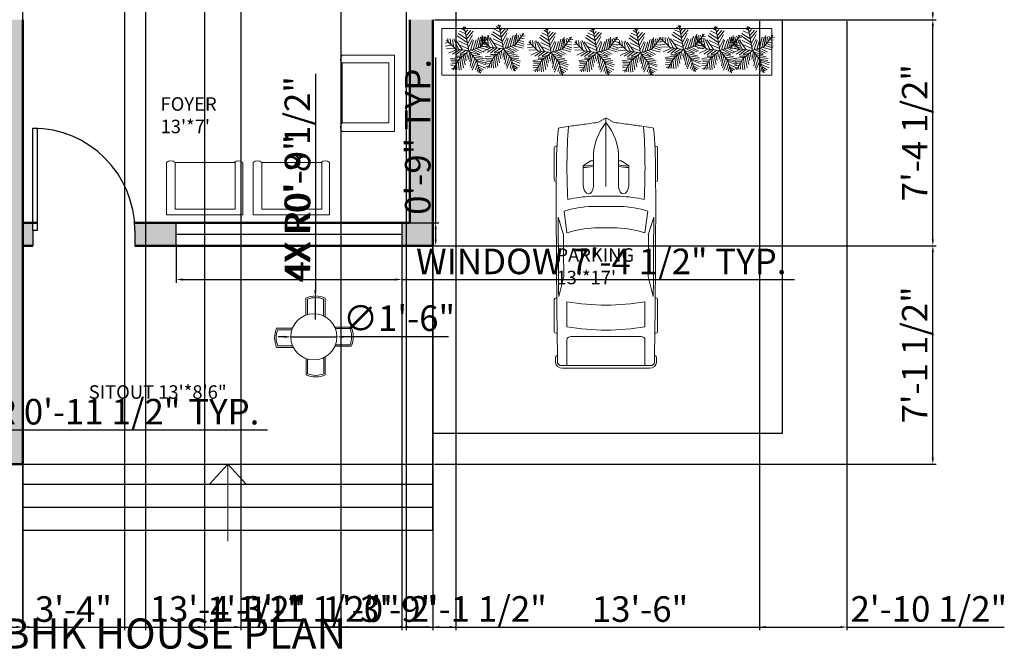
# Model space of a CAD drawing. Units: inches. Extents: x 772 to 1415, y 1573 to 2261.
# Tile 2 of 4: x 984 to 1369, y 1573 to 1820. Entities that reach past the tile are written whole.
import ezdxf

# ---------------------------------------------------------------- set-up
doc = ezdxf.new("R2010")
doc.units = ezdxf.units.IN
for name, color, linetype, lineweight in [('A-ANNO-DIMS', 2, 'Continuous', 18), ('A-ANNO-SYMB', 7, 'Continuous', 18), ('A-ANNO-TEXT', 10, 'Continuous', 25), ('A-AREA-IDEN', 10, 'Continuous', 25), ('A-EQPM-VEH', 8, 'Continuous', 13), ('A-FLOR-EDGE', 7, 'Continuous', 25), ('A-FLOR-STRS', 7, 'Continuous', 25), ('A-WALL-PATT', 140, 'Continuous', 13), ('DOOR', 52, 'Continuous', 25), ('FUR', 210, 'Continuous', 18), ('L-PLNT-BEDS', 92, 'Continuous', 18), ('TREE', 92, 'Continuous', 13), ('WALL', 7, 'Continuous', 50), ('WINDOW', 80, 'Continuous', 25)]:
    doc.layers.add(name, color=color, linetype=linetype, lineweight=lineweight)
doc.styles.get("Standard").update_dxf_attribs({"font": 'arial.ttf'})
doc.dimstyles.new('ISO-25', dxfattribs={"dimtxt": 10, "dimasz": 2.5, "dimexe": 1.25, "dimexo": 0.625, "dimtad": 1, "dimdec": 0, "dimlunit": 4, "dimtxsty": 'Standard', "dimcen": 2.5, "dimadec": 0, "dimazin": 0, "dimtfac": 1, "dimtdec": 0, "dimtmove": 0, "dimatfit": 3, "dimfxl": 1, "dimarcsym": 0})

# ---------------------------------------------------------------- blocks, each defined once
blk = doc.blocks.new('*U2')
for p, q in [((0, 0), (0, -6)), ((40, 0), (40, -6))]:
    blk.add_line(p, q)
blk.add_lwpolyline([(0, 0), (0, 40), (1.75, 40), (1.75, 0)], close=True)
blk.add_arc((0, 0), 40, 0, 90)
blk = doc.blocks.new('*U6')
for p, q in [((-7.288, 39.707), (-21.778, 46.673)), ((-8.737, 47.138), (-17.069, 52.711)), ((-10.186, 53.64), (-13.084, 55.962)), ((0, 0), (-10.5, 57)), ((-9.099, 51.782), (-6.563, 55.962)), ((-7.65, 43.423), (-2.578, 49.46)), ((-5.839, 35.992), (4.667, 48.067)), ((-5.114, 27.632), (10.463, 46.673)), ((-31.5, 4.5), (-52.5, 25.5)), ((-48.585, 21.131), (-49.309, 29.026)), ((-43.513, 28.561), (-42.427, 15.558)), ((-38.442, 26.239), (-34.819, 7.663)), ((-35.544, 28.097), (-24.314, 3.947)), ((-14.533, 2.09), (-30.834, 25.31)), ((-3.665, 19.273), (-27.574, 35.527)), ((-5.114, 28.097), (-24.676, 40.636)), ((-24.314, 23.917), (-2.941, 13.7)), ((-2.941, 16.486), (8.652, 37.85)), ((-1.129, 6.734), (9.014, 26.704)), ((3.942, 1.625), (11.187, 24.381)), ((10.101, 3.483), (17.708, 26.239)), ((16.259, 5.805), (23.142, 31.348)), ((22.055, 7.198), (27.489, 32.277)), ((27, 9), (48, 36)), ((27.127, 9.056), (31.112, 35.992)), ((31.836, 30.883), (32.561, 16.486)), ((35.096, 32.741), (37.27, 22.524)), ((38.719, 34.134), (41.979, 28.561)), ((40.53, 25.775), (48.862, 24.846)), ((43.791, 29.954), (51.036, 30.883)), ((44.153, 36.456), (45.239, 32.741)), ((-47.498, 19.737), (-55.83, 18.344)), ((-40.615, 13.7), (-55.105, 10.913)), ((-33.37, 6.269), (-52.207, 5.34)), ((-28.299, 3.483), (-47.86, -5.805)), ((-21.416, 3.018), (-38.079, -8.128)), ((0, 0), (-31.5, 4.5)), ((-15.982, 2.09), (-30.11, -9.521)), ((0, 0), (-22.5, -19.5)), ((-6.563, 1.161), (-21.416, -8.128)), ((-20.691, 13.7), (-1.129, 4.876)), ((0, 0), (27, 9)), ((0, 0), (18, -22.5)), ((6.478, 1.625), (26.04, -8.592)), ((11.187, 3.483), (30.749, -5.805)), ((18.07, 5.805), (35.096, -3.483)), ((24.229, 7.663), (46.688, 1.625)), ((29.662, 12.307), (48.137, 6.269)), ((33.285, 16.486), (48.862, 10.913)), ((36.183, 19.737), (48.137, 17.88)), ((-17.431, -15.094), (-42.789, -18.809)), ((-24.314, -21.596), (-42.427, -22.06)), ((-22.5, -19.5), (-37.5, -45)), ((-15.257, -12.772), (-30.11, -12.772)), ((-20.691, -18.345), (-17.793, -44.352)), ((-6.563, -5.805), (-19.967, -9.985)), ((-17.069, -15.094), (-12.721, -40.172)), ((-13.446, -11.378), (-8.737, -32.741)), ((-9.461, -8.592), (-6.201, -23.453)), ((-4.752, -3.483), (-3.665, -14.629)), ((2.493, -3.019), (-1.491, -20.202)), ((1.769, -2.555), (24.229, -9.521)), ((5.029, -6.27), (2.131, -25.775)), ((9.014, -11.378), (3.58, -35.992)), ((14.085, -16.951), (6.478, -40.172)), ((7.565, -9.056), (32.198, -14.629)), ((18.07, -22.524), (8.289, -45.745)), ((12.274, -15.094), (36.907, -18.809)), ((16.259, -19.738), (36.183, -22.989)), ((18, -22.5), (27, -52.5)), ((18.433, -22.524), (40.53, -29.026)), ((-28.299, -29.026), (-42.789, -31.348)), ((-30.834, -34.135), (-42.427, -35.528)), ((-34.457, -39.708), (-40.978, -42.494)), ((-26.849, -26.24), (-40.253, -25.775)), ((-32.646, -36.921), (-31.921, -44.352)), ((-29.023, -30.884), (-27.936, -43.887)), ((-25.038, -23.918), (-22.865, -45.281)), ((20.244, -30.419), (15.897, -44.816)), ((19.157, -25.311), (38.719, -33.206)), ((22.78, -37.85), (19.519, -48.532)), ((21.331, -32.741), (39.081, -40.636)), ((22.78, -38.314), (34.372, -44.816)), ((24.591, -45.745), (23.142, -50.854)), ((24.591, -43.423), (30.749, -47.603)), ((26.764, -49.925), (28.213, -50.854))]:
    blk.add_line(p, q)
blk = doc.blocks.new('*U8')
for p, q in [((21.1, 37.41), (21.1, 36.83)), ((46.55, 38.89), (22.35, 38.89)), ((47.8, 37.39), (47.8, 37.41)), ((135.45, 37.07), (135.45, 37.41)), ((136.7, 38.89), (160.9, 38.89)), ((162.15, 37.41), (162.15, 36.77)), ((70.03, 31.54), (86.41, 29.35)), ((87.99, 31.87), (74.76, 35.92)), ((134.31, 35.6), (119.29, 31.78)), ((186.47, -33.5), (186.47, 33.5)), ((188.4, -32.76), (188.4, 32.76)), ((138.42, 29.35), (157.25, 29.35)), ((164.52, 26.39), (164.52, -26.39)), ((186.47, 29.35), (167.01, 29.35)), ((32.27, 11.63), (36.13, 17.17)), ((36.13, 17.17), (50.94, 17.17)), ((29.77, 9.51), (51.68, 9.51)), ((32.12, 9.51), (32.12, 11.15)), ((58.92, -10.77), (58.92, 10.77)), ((66.55, -10.53), (66.55, 10.53)), ((82.74, 8.5), (82.74, -8.5)), ((186.47, -10.53), (186.47, 10.53)), ((3.27, 6.13), (0.1, 0.41)), ((0, 0), (51.68, 0)), ((0.1, -0.41), (3.27, -6.13)), ((29.77, -9.51), (51.68, -9.51)), ((32.12, -9.51), (32.12, -11.15)), ((32.27, -11.63), (36.13, -17.17)), ((36.13, -17.17), (50.94, -17.17)), ((86.41, -29.35), (70.03, -31.54)), ((157.25, -29.35), (138.42, -29.35)), ((167.01, -29.35), (186.47, -29.35)), ((21.1, -37.41), (21.1, -36.83)), ((87.99, -31.87), (74.76, -35.92)), ((134.31, -35.6), (119.29, -31.78)), ((162.15, -37.41), (162.15, -36.77)), ((46.55, -38.89), (22.35, -38.89)), ((47.8, -37.39), (47.8, -37.41)), ((135.45, -37.07), (135.45, -37.41)), ((136.7, -38.89), (160.9, -38.89))]:
    blk.add_line(p, q)
for centre, major_axis, ratio, start_param, end_param in [((41.19, -490.86), (0, 528.23), 0.842304, 0.00281, 0.075598), ((22.35, 37.41), (0, -1.48), 0.842304, 3.141593, 4.712389), ((64.48, -10555.62), (0, 10593.03), 0.842304, -0.013397, 0.002797), ((46.55, 37.41), (0, 1.48), 0.842304, -1.570796, 0), ((136.7, 37.41), (0, -1.48), 0.842304, 3.141593, 4.712389), ((160.9, 37.41), (0, 1.48), 0.842304, -1.570796, 0), ((180.63, 35.84), (0, 2.22), 0.842304, -0.013017, 1.249894), ((64.48, -10556.36), (0, 10595.31), 0.842304, -0.013397, -0.013017), ((183.98, 32.76), (0, -5.25), 0.842304, 1.570796, 3.128196), ((266.03, -27.52), (0, 313.31), 0.842304, 1.367076, 1.39176), ((37.47, -593.96), (0, -623.33), 0.842304, 3.096046, 3.200911), ((135.29, 5.39), (0, 81.77), 0.842304, 1.245306, 1.50788), ((64.48, -10555.62), (0, -10591.55), 0.842304, 3.133765, 3.140441), ((95.79, -3666.35), (0, -3698.24), 0.842304, 3.134049, 3.144098), ((183.98, 33.5), (0, -2.96), 0.842304, 1.570796, 3.128196), ((259.18, -27.52), (0, -305.3), 0.842304, 4.528606, 4.561838), ((134.4, 5.39), (0, -89.78), 0.842304, 4.449482, 4.652344), ((149.6, 2.8), (0, -79.58), 0.842304, 4.372215, 4.640744), ((17.08, 0), (0, 147.02), 0.842304, 4.511394, 4.913384), ((35.91, 0), (0, 147.02), 0.842304, 4.511394, 4.913384), ((167.01, 26.39), (0, 2.96), 0.842304, 0, 1.570796), ((-204.49, 52.4), (0, -250.96), 0.842304, 1.385369, 1.434372), ((13.04, 17.01), (0, 27.42), 0.842304, 4.435146, 4.718221), ((14.2, 17.01), (0, 27.42), 0.842304, 4.435146, 4.718221), ((50.79, 13.34), (6.34, -0.36), 0.603834, -1.395552, 1.581315), ((29.77, -46.66), (0, 56.17), 0.842304, 0, 0.590319), ((32.75, 11.15), (0, 0.74), 0.842304, 0.879714, 1.570796), ((0.62, 0), (0, -0.74), 0.842304, 4.131459, 5.293319), ((-204.49, -52.4), (0, 250.96), 0.842304, -1.434372, -1.385369), ((29.77, 46.66), (0, 56.17), 0.842304, 2.551274, 3.141593), ((32.75, -11.15), (0, -0.74), 0.842304, 4.712389, 5.403472), ((13.04, -17.01), (0, -27.42), 0.842304, 1.564964, 1.848039), ((14.2, -17.01), (0, -27.42), 0.842304, 1.564964, 1.848039), ((134.4, -5.39), (0, -89.78), 0.842304, -1.510751, -1.307889), ((135.29, -5.39), (0, -81.77), 0.842304, -1.50788, -1.245306), ((149.6, -2.8), (0, -79.58), 0.842304, -1.499151, -1.230623), ((259.18, 27.52), (0, 305.3), 0.842304, 1.721348, 1.754579), ((266.03, 27.52), (0, 313.31), 0.842304, 1.749832, 1.774517), ((37.47, 593.96), (0, -623.33), 0.842304, -0.059319, 0.045547), ((167.01, -26.39), (0, -2.96), 0.842304, 4.712389, 6.283185), ((41.19, 490.86), (0, -528.23), 0.842304, -0.075598, -0.00281), ((64.48, 10555.62), (0, 10593.03), 0.842304, 3.138796, 3.15499), ((64.48, 10555.62), (0, -10591.55), 0.842304, 0.001152, 0.007828), ((95.79, 3666.35), (0, -3698.24), 0.842304, -0.002505, 0.007544), ((180.63, -35.84), (0, -2.22), 0.842304, -1.249894, 0.013017), ((183.98, -33.5), (0, 2.96), 0.842304, 3.15499, 4.712389), ((183.98, -32.76), (0, -5.25), 0.842304, 0.013397, 1.570796), ((22.35, -37.41), (0, 1.48), 0.842304, 1.570796, 3.141593), ((46.55, -37.41), (0, -1.48), 0.842304, 0, 1.570796), ((136.7, -37.41), (0, -1.48), 0.842304, -1.570796, 0), ((160.9, -37.41), (0, 1.48), 0.842304, 3.141593, 4.712389), ((64.48, 10556.36), (0, 10595.31), 0.842304, 3.15461, 3.15499)]:
    blk.add_ellipse(centre, major_axis=major_axis, ratio=ratio, start_param=start_param, end_param=end_param)
at = {"extrusion": (0, 0, -1)}
blk.add_ellipse((50.79, -13.34), major_axis=(6.34, 0.36), ratio=0.603834, start_param=-1.395552, end_param=1.581315, dxfattribs=at)
blk = doc.blocks.new('CHAIR-LOUNGE')
for p, q in [((0, 20.45), (0, 0)), ((26.89, 20.45), (26.11, 20.45)), ((29.8, 0), (29.8, 20.45)), ((0, 0), (29.8, 0))]:
    blk.add_line(p, q)
blk.add_lwpolyline([(3.35, 2.16), (26.89, 2.16), (26.89, 20.45), (3.35, 20.45)], close=True)
for centre in [(1.67, 18.73), (28.12, 18.73)]:
    blk.add_arc(centre, 2.4, 45.7795, 134.2205)
blk = doc.blocks.new('WIN-88IN')
blk.add_line((0, 4.5), (88.26, 4.5))
blk.add_lwpolyline([(0, 9), (88.26, 9), (88.26, 0), (0, 0)], close=True)
blk = doc.blocks.new('*D27')
at = {"layer": 'A-ANNO-DIMS', "color": 0, "lineweight": -2, "transparency": 16777216}
for p, q in [((1037.11, 1828.64), (1037.11, 1823.55)), ((1066.91, 1828.64), (1066.91, 1823.55)), ((1039.61, 1824.8), (1064.41, 1824.8)), ((1066.91, 1824.8), (1241.4, 1824.8))]:
    blk.add_line(p, q, dxfattribs=at)
at = {"layer": 'A-ANNO-DIMS', "color": 0, "transparency": 16777216}
for points in [[(1039.61, 1825.21), (1039.61, 1824.38), (1037.11, 1824.8)], [(1064.41, 1825.21), (1064.41, 1824.38), (1066.91, 1824.8)]]:
    blk.add_solid(points, dxfattribs=at)
at = {"layer": 'Defpoints', "color": 0, "transparency": 16777216}
for p in [(1037.11, 1829.27), (1066.91, 1829.27), (1066.91, 1824.8)]:
    blk.add_point(p, dxfattribs=at)
at = {"layer": 'A-ANNO-DIMS', "color": 0, "transparency": 16777216, "insert": (1155.4, 1830.59), "char_height": 10, "attachment_point": 5}
blk.add_mtext('LOUNGE CHAIR 2\'-6" TYP.', dxfattribs=at)
blk = doc.blocks.new('*D37')
at = {"layer": 'A-ANNO-DIMS', "color": 0, "lineweight": -2, "transparency": 16777216}
for p, q in [((1045.2, 1730.86), (1045.2, 1716.99)), ((1133.46, 1730.86), (1133.46, 1716.99)), ((1047.7, 1718.24), (1130.96, 1718.24)), ((1133.46, 1718.24), (1287.06, 1718.24))]:
    blk.add_line(p, q, dxfattribs=at)
at = {"layer": 'A-ANNO-DIMS', "color": 0, "transparency": 16777216}
for points in [[(1047.7, 1718.66), (1047.7, 1717.83), (1045.2, 1718.24)], [(1130.96, 1718.66), (1130.96, 1717.83), (1133.46, 1718.24)]]:
    blk.add_solid(points, dxfattribs=at)
at = {"layer": 'Defpoints', "color": 0, "transparency": 16777216}
for p in [(1045.2, 1731.48), (1133.46, 1731.48), (1133.46, 1718.24)]:
    blk.add_point(p, dxfattribs=at)
at = {"layer": 'A-ANNO-DIMS', "color": 0, "transparency": 16777216, "insert": (1211.51, 1724.04), "char_height": 10, "attachment_point": 5}
blk.add_mtext('WINDOW 7\'-4 1/2" TYP.', dxfattribs=at)
blk = doc.blocks.new('*D38')
at = {"layer": 'A-ANNO-DIMS', "color": 0, "lineweight": -2, "transparency": 16777216}
for p, q in [((1146.7, 1740.48), (1146.7, 1805.19)), ((1134.09, 1740.48), (1147.95, 1740.48)), ((1146.7, 1733.98), (1146.7, 1737.98)), ((1134.09, 1731.48), (1147.95, 1731.48))]:
    blk.add_line(p, q, dxfattribs=at)
at = {"layer": 'A-ANNO-DIMS', "color": 0, "transparency": 16777216}
for points in [[(1146.29, 1737.98), (1147.12, 1737.98), (1146.7, 1740.48)], [(1146.29, 1733.98), (1147.12, 1733.98), (1146.7, 1731.48)]]:
    blk.add_solid(points, dxfattribs=at)
at = {"layer": 'Defpoints', "color": 0, "transparency": 16777216}
for p in [(1133.46, 1740.48), (1146.7, 1740.48), (1133.46, 1731.48)]:
    blk.add_point(p, dxfattribs=at)
at = {"layer": 'A-ANNO-DIMS', "color": 0, "transparency": 16777216, "insert": (1140.97, 1774.09), "char_height": 10, "attachment_point": 5, "rotation": 90}
blk.add_mtext('0\'-9" TYP.', dxfattribs=at)
blk = doc.blocks.new('*D39')
at = {"layer": 'A-ANNO-DIMS', "color": 0, "lineweight": -2, "transparency": 16777216}
for p, q in [((911.44, 1660.47), (911.44, 1658.15)), ((913.94, 1659.4), (920.23, 1659.4)), ((922.73, 1660.47), (922.73, 1658.15)), ((922.73, 1659.4), (1080.94, 1659.4))]:
    blk.add_line(p, q, dxfattribs=at)
at = {"layer": 'A-ANNO-DIMS', "color": 0, "transparency": 16777216}
for points in [[(913.94, 1659.82), (913.94, 1658.99), (911.44, 1659.4)], [(920.23, 1659.82), (920.23, 1658.99), (922.73, 1659.4)]]:
    blk.add_solid(points, dxfattribs=at)
at = {"layer": 'Defpoints', "color": 0, "transparency": 16777216}
for p in [(911.44, 1661.1), (922.73, 1661.1), (922.73, 1659.4)]:
    blk.add_point(p, dxfattribs=at)
at = {"layer": 'A-ANNO-DIMS', "color": 0, "transparency": 16777216, "insert": (1003.09, 1665.2), "char_height": 10, "attachment_point": 5}
blk.add_mtext('BURNER 0\'-11 1/2" TYP.', dxfattribs=at)
blk = doc.blocks.new('*D41')
at = {"layer": 'A-ANNO-DIMS', "color": 0, "lineweight": -2, "transparency": 16777216}
for p, q in [((827.65, 1645.36), (827.65, 1580.94)), ((985.15, 1645.36), (985.15, 1580.94)), ((830.15, 1582.19), (982.65, 1582.19))]:
    blk.add_line(p, q, dxfattribs=at)
at = {"layer": 'A-ANNO-DIMS', "color": 0, "transparency": 16777216}
for points in [[(830.15, 1582.61), (830.15, 1581.78), (827.65, 1582.19)], [(982.65, 1582.61), (982.65, 1581.78), (985.15, 1582.19)]]:
    blk.add_solid(points, dxfattribs=at)
at = {"layer": 'Defpoints', "color": 0, "transparency": 16777216}
for p in [(827.65, 1645.98), (985.15, 1645.98), (985.15, 1582.19)]:
    blk.add_point(p, dxfattribs=at)
at = {"layer": 'A-ANNO-DIMS', "color": 0, "transparency": 16777216, "insert": (906.4, 1587.99), "char_height": 10, "attachment_point": 5}
blk.add_mtext('13\'-1 1/2"', dxfattribs=at)
blk = doc.blocks.new('*D42')
at = {"layer": 'A-ANNO-DIMS', "color": 0, "lineweight": -2, "transparency": 16777216}
for p, q in [((985.15, 1645.36), (985.15, 1580.94)), ((1145.65, 1645.36), (1145.65, 1580.94)), ((987.65, 1582.19), (1143.15, 1582.19))]:
    blk.add_line(p, q, dxfattribs=at)
at = {"layer": 'A-ANNO-DIMS', "color": 0, "transparency": 16777216}
for points in [[(987.65, 1582.61), (987.65, 1581.78), (985.15, 1582.19)], [(1143.15, 1582.61), (1143.15, 1581.78), (1145.65, 1582.19)]]:
    blk.add_solid(points, dxfattribs=at)
at = {"layer": 'Defpoints', "color": 0, "transparency": 16777216}
for p in [(985.15, 1645.98), (1145.65, 1645.98), (1145.65, 1582.19)]:
    blk.add_point(p, dxfattribs=at)
at = {"layer": 'A-ANNO-DIMS', "color": 0, "transparency": 16777216, "insert": (1065.4, 1587.99), "char_height": 10, "attachment_point": 5}
blk.add_mtext('13\'-4 1/2"', dxfattribs=at)
blk = doc.blocks.new('*D43')
at = {"layer": 'A-ANNO-DIMS', "color": 0, "lineweight": -2, "transparency": 16777216}
for p, q in [((1307.65, 1819.36), (1307.65, 1580.94)), ((1145.65, 1645.36), (1145.65, 1580.94)), ((1148.15, 1582.19), (1305.15, 1582.19))]:
    blk.add_line(p, q, dxfattribs=at)
at = {"layer": 'A-ANNO-DIMS', "color": 0, "transparency": 16777216}
for points in [[(1148.15, 1582.61), (1148.15, 1581.78), (1145.65, 1582.19)], [(1305.15, 1582.61), (1305.15, 1581.78), (1307.65, 1582.19)]]:
    blk.add_solid(points, dxfattribs=at)
at = {"layer": 'Defpoints', "color": 0, "transparency": 16777216}
for p in [(1307.65, 1819.98), (1145.65, 1645.98), (1307.65, 1582.19)]:
    blk.add_point(p, dxfattribs=at)
at = {"layer": 'A-ANNO-DIMS', "color": 0, "transparency": 16777216, "insert": (1226.65, 1587.93), "char_height": 10, "attachment_point": 5}
blk.add_mtext('13\'-6"', dxfattribs=at)
blk = doc.blocks.new('*D44')
at = {"layer": 'A-ANNO-DIMS', "color": 0, "lineweight": -2, "transparency": 16777216}
for p, q in [((1146.28, 1731.48), (1342.5, 1731.48)), ((1341.25, 1648.48), (1341.25, 1728.98)), ((1146.28, 1645.98), (1342.5, 1645.98))]:
    blk.add_line(p, q, dxfattribs=at)
at = {"layer": 'A-ANNO-DIMS', "color": 0, "transparency": 16777216}
for points in [[(1340.83, 1728.98), (1341.67, 1728.98), (1341.25, 1731.48)], [(1340.83, 1648.48), (1341.67, 1648.48), (1341.25, 1645.98)]]:
    blk.add_solid(points, dxfattribs=at)
at = {"layer": 'Defpoints', "color": 0, "transparency": 16777216}
for p in [(1145.65, 1731.48), (1341.25, 1731.48), (1145.65, 1645.98)]:
    blk.add_point(p, dxfattribs=at)
at = {"layer": 'A-ANNO-DIMS', "color": 0, "transparency": 16777216, "insert": (1335.46, 1688.73), "char_height": 10, "attachment_point": 5, "rotation": 90}
blk.add_mtext('7\'-1 1/2"', dxfattribs=at)
blk = doc.blocks.new('*D45')
at = {"layer": 'A-ANNO-DIMS', "color": 0, "lineweight": -2, "transparency": 16777216}
for p, q in [((1146.28, 1819.98), (1342.5, 1819.98)), ((1341.25, 1733.98), (1341.25, 1817.48)), ((1146.28, 1731.48), (1342.5, 1731.48))]:
    blk.add_line(p, q, dxfattribs=at)
at = {"layer": 'A-ANNO-DIMS', "color": 0, "transparency": 16777216}
for points in [[(1340.83, 1817.48), (1341.67, 1817.48), (1341.25, 1819.98)], [(1340.83, 1733.98), (1341.67, 1733.98), (1341.25, 1731.48)]]:
    blk.add_solid(points, dxfattribs=at)
at = {"layer": 'Defpoints', "color": 0, "transparency": 16777216}
for p in [(1145.65, 1819.98), (1341.25, 1819.98), (1145.65, 1731.48)]:
    blk.add_point(p, dxfattribs=at)
at = {"layer": 'A-ANNO-DIMS', "color": 0, "transparency": 16777216, "insert": (1335.46, 1775.73), "char_height": 10, "attachment_point": 5, "rotation": 90}
blk.add_mtext('7\'-4 1/2"', dxfattribs=at)
blk = doc.blocks.new('*D46')
at = {"layer": 'A-ANNO-DIMS', "color": 0, "lineweight": -2, "transparency": 16777216}
for p, q in [((1299.28, 2004.48), (1342.5, 2004.48)), ((1341.25, 1822.48), (1341.25, 2001.98)), ((1308.28, 1819.98), (1342.5, 1819.98))]:
    blk.add_line(p, q, dxfattribs=at)
at = {"layer": 'A-ANNO-DIMS', "color": 0, "transparency": 16777216}
for points in [[(1340.83, 2001.98), (1341.67, 2001.98), (1341.25, 2004.48)], [(1340.83, 1822.48), (1341.67, 1822.48), (1341.25, 1819.98)]]:
    blk.add_solid(points, dxfattribs=at)
at = {"layer": 'Defpoints', "color": 0, "transparency": 16777216}
for p in [(1298.65, 2004.48), (1341.25, 2004.48), (1307.65, 1819.98)]:
    blk.add_point(p, dxfattribs=at)
at = {"layer": 'A-ANNO-DIMS', "color": 0, "transparency": 16777216, "insert": (1335.46, 1912.23), "char_height": 10, "attachment_point": 5, "rotation": 90}
blk.add_mtext('15\'-4 1/2"', dxfattribs=at)
blk = doc.blocks.new('*D55')
at = {"layer": 'A-ANNO-DIMS', "color": 0, "lineweight": -2, "transparency": 16777216}
for p, q in [((1273.39, 1819.36), (1273.39, 1580.94)), ((1307.65, 1819.36), (1307.65, 1580.94)), ((1275.89, 1582.19), (1305.15, 1582.19)), ((1307.65, 1582.19), (1369.22, 1582.19))]:
    blk.add_line(p, q, dxfattribs=at)
at = {"layer": 'A-ANNO-DIMS', "color": 0, "transparency": 16777216}
for points in [[(1275.89, 1582.61), (1275.89, 1581.78), (1273.39, 1582.19)], [(1305.15, 1582.61), (1305.15, 1581.78), (1307.65, 1582.19)]]:
    blk.add_solid(points, dxfattribs=at)
at = {"layer": 'Defpoints', "color": 0, "transparency": 16777216}
for p in [(1273.39, 1819.98), (1307.65, 1819.98), (1307.65, 1582.19)]:
    blk.add_point(p, dxfattribs=at)
at = {"layer": 'A-ANNO-DIMS', "color": 0, "transparency": 16777216, "insert": (1339.69, 1587.99), "char_height": 10, "attachment_point": 5}
blk.add_mtext('2\'-10 1/2"', dxfattribs=at)
blk = doc.blocks.new('*D56')
at = {"layer": 'A-ANNO-DIMS', "color": 0, "lineweight": -2, "transparency": 16777216}
for p, q in [((1133.46, 1730.86), (1133.46, 1580.94)), ((1145.65, 1730.86), (1145.65, 1580.94)), ((1133.46, 1582.19), (1104.07, 1582.19)), ((1143.15, 1582.19), (1135.96, 1582.19))]:
    blk.add_line(p, q, dxfattribs=at)
at = {"layer": 'A-ANNO-DIMS', "color": 0, "transparency": 16777216}
for points in [[(1135.96, 1582.61), (1135.96, 1581.78), (1133.46, 1582.19)], [(1143.15, 1582.61), (1143.15, 1581.78), (1145.65, 1582.19)]]:
    blk.add_solid(points, dxfattribs=at)
at = {"layer": 'Defpoints', "color": 0, "transparency": 16777216}
for p in [(1133.46, 1731.48), (1145.65, 1731.48), (1133.46, 1582.19)]:
    blk.add_point(p, dxfattribs=at)
at = {"layer": 'A-ANNO-DIMS', "color": 0, "transparency": 16777216, "insert": (1117.52, 1587.92), "char_height": 10, "attachment_point": 5}
blk.add_mtext('1\'-0"', dxfattribs=at)
blk = doc.blocks.new('*D59')
at = {"layer": 'A-ANNO-DIMS', "color": 0, "lineweight": -2, "transparency": 16777216}
for p, q in [((1109.65, 2003.86), (1109.65, 1580.94)), ((1154.65, 2003.86), (1154.65, 1580.94)), ((1112.15, 1582.19), (1152.15, 1582.19))]:
    blk.add_line(p, q, dxfattribs=at)
at = {"layer": 'A-ANNO-DIMS', "color": 0, "transparency": 16777216}
for points in [[(1112.15, 1582.61), (1112.15, 1581.78), (1109.65, 1582.19)], [(1152.15, 1582.61), (1152.15, 1581.78), (1154.65, 1582.19)]]:
    blk.add_solid(points, dxfattribs=at)
at = {"layer": 'Defpoints', "color": 0, "transparency": 16777216}
for p in [(1109.65, 2004.48), (1154.65, 2004.48), (1154.65, 1582.19)]:
    blk.add_point(p, dxfattribs=at)
at = {"layer": 'A-ANNO-DIMS', "color": 0, "transparency": 16777216, "insert": (1132.15, 1587.93), "char_height": 10, "attachment_point": 5}
blk.add_mtext('3\'-9"', dxfattribs=at)
blk = doc.blocks.new('*D60')
at = {"layer": 'A-ANNO-DIMS', "color": 0, "lineweight": -2, "transparency": 16777216}
for p, q in [((984.95, 2003.86), (984.95, 1580.94)), ((1024.95, 2003.86), (1024.95, 1580.94)), ((987.45, 1582.19), (1022.45, 1582.19))]:
    blk.add_line(p, q, dxfattribs=at)
at = {"layer": 'A-ANNO-DIMS', "color": 0, "transparency": 16777216}
for points in [[(987.45, 1582.61), (987.45, 1581.78), (984.95, 1582.19)], [(1022.45, 1582.61), (1022.45, 1581.78), (1024.95, 1582.19)]]:
    blk.add_solid(points, dxfattribs=at)
at = {"layer": 'Defpoints', "color": 0, "transparency": 16777216}
for p in [(984.95, 2004.48), (1024.95, 2004.48), (1024.95, 1582.19)]:
    blk.add_point(p, dxfattribs=at)
at = {"layer": 'A-ANNO-DIMS', "color": 0, "transparency": 16777216, "insert": (1004.95, 1587.93), "char_height": 10, "attachment_point": 5}
blk.add_mtext('3\'-4"', dxfattribs=at)
blk = doc.blocks.new('*D61')
at = {"layer": 'A-ANNO-DIMS', "color": 0, "lineweight": -2, "transparency": 16777216}
for p, q in [((1056.25, 2011.79), (1056.25, 1580.94)), ((1033.15, 2008.36), (1033.15, 1580.94)), ((1035.65, 1582.19), (1053.75, 1582.19)), ((1056.25, 1582.19), (1093.41, 1582.19))]:
    blk.add_line(p, q, dxfattribs=at)
at = {"layer": 'A-ANNO-DIMS', "color": 0, "transparency": 16777216}
for points in [[(1035.65, 1582.61), (1035.65, 1581.78), (1033.15, 1582.19)], [(1053.75, 1582.61), (1053.75, 1581.78), (1056.25, 1582.19)]]:
    blk.add_solid(points, dxfattribs=at)
at = {"layer": 'Defpoints', "color": 0, "transparency": 16777216}
for p in [(1056.25, 2012.41), (1033.15, 2008.98), (1056.25, 1582.19)]:
    blk.add_point(p, dxfattribs=at)
at = {"layer": 'A-ANNO-DIMS', "color": 0, "transparency": 16777216, "insert": (1076.08, 1587.84), "char_height": 10, "attachment_point": 5}
blk.add_mtext('1\'-11"', dxfattribs=at)
blk = doc.blocks.new('*D62')
at = {"layer": 'A-ANNO-DIMS', "color": 0, "lineweight": -2, "transparency": 16777216}
for p, q in [((1033.15, 2092.36), (1033.15, 1580.94)), ((1070.44, 2092.36), (1070.44, 1580.94)), ((1035.65, 1582.19), (1067.94, 1582.19)), ((1070.44, 1582.19), (1124.06, 1582.19))]:
    blk.add_line(p, q, dxfattribs=at)
at = {"layer": 'A-ANNO-DIMS', "color": 0, "transparency": 16777216}
for points in [[(1035.65, 1582.61), (1035.65, 1581.78), (1033.15, 1582.19)], [(1067.94, 1582.61), (1067.94, 1581.78), (1070.44, 1582.19)]]:
    blk.add_solid(points, dxfattribs=at)
at = {"layer": 'Defpoints', "color": 0, "transparency": 16777216}
for p in [(1033.15, 2092.98), (1070.44, 2092.98), (1070.44, 1582.19)]:
    blk.add_point(p, dxfattribs=at)
at = {"layer": 'A-ANNO-DIMS', "color": 0, "transparency": 16777216, "insert": (1098.5, 1587.99), "char_height": 10, "attachment_point": 5}
blk.add_mtext('3\'-1 1/2"', dxfattribs=at)
blk = doc.blocks.new('*D63')
at = {"layer": 'A-ANNO-DIMS', "color": 0, "lineweight": -2, "transparency": 16777216}
for p, q in [((1109.65, 2099.86), (1109.65, 1580.94)), ((1135.17, 2099.86), (1135.17, 1580.94)), ((1112.15, 1582.19), (1132.67, 1582.19)), ((1135.17, 1582.19), (1188.98, 1582.19))]:
    blk.add_line(p, q, dxfattribs=at)
at = {"layer": 'A-ANNO-DIMS', "color": 0, "transparency": 16777216}
for points in [[(1112.15, 1582.61), (1112.15, 1581.78), (1109.65, 1582.19)], [(1132.67, 1582.61), (1132.67, 1581.78), (1135.17, 1582.19)]]:
    blk.add_solid(points, dxfattribs=at)
at = {"layer": 'Defpoints', "color": 0, "transparency": 16777216}
for p in [(1109.65, 2100.48), (1135.17, 2100.48), (1135.17, 1582.19)]:
    blk.add_point(p, dxfattribs=at)
at = {"layer": 'A-ANNO-DIMS', "color": 0, "transparency": 16777216, "insert": (1163.33, 1587.99), "char_height": 10, "attachment_point": 5}
blk.add_mtext('2\'-1 1/2"', dxfattribs=at)
blk = doc.blocks.new('*D64')
at = {"layer": 'A-ANNO-DIMS', "color": 0, "lineweight": -2, "transparency": 16777216}
for p, q in [((1099.66, 1776.1), (1099.66, 1714.31)), ((1099.66, 1702.63), (1099.66, 1711.81))]:
    blk.add_line(p, q, dxfattribs=at)
at = {"layer": 'A-ANNO-DIMS', "color": 0, "transparency": 16777216}
blk.add_solid([(1099.24, 1714.31), (1100.07, 1714.31), (1099.66, 1711.81)], dxfattribs=at)
at = {"layer": 'Defpoints', "color": 0, "transparency": 16777216}
for p in [(1099.66, 1711.81), (1099.66, 1702.63)]:
    blk.add_point(p, dxfattribs=at)
at = {"layer": 'A-ANNO-DIMS', "color": 0, "transparency": 16777216, "insert": (1093.93, 1746.45), "char_height": 10, "attachment_point": 5, "rotation": 89.9987}
blk.add_mtext('4X R0\'-9"', dxfattribs=at)
blk = doc.blocks.new('*D65')
at = {"layer": 'A-ANNO-DIMS', "color": 0, "lineweight": -2, "transparency": 16777216}
for p, q in [((1099.66, 1798.77), (1099.66, 1713.67)), ((1099.66, 1702.63), (1099.66, 1711.17))]:
    blk.add_line(p, q, dxfattribs=at)
at = {"layer": 'A-ANNO-DIMS', "color": 0, "transparency": 16777216}
blk.add_solid([(1099.24, 1713.67), (1100.07, 1713.67), (1099.66, 1711.17)], dxfattribs=at)
at = {"layer": 'Defpoints', "color": 0, "transparency": 16777216}
for p in [(1099.66, 1711.17), (1099.66, 1702.63)]:
    blk.add_point(p, dxfattribs=at)
at = {"layer": 'A-ANNO-DIMS', "color": 0, "transparency": 16777216, "insert": (1093.86, 1757.47), "char_height": 10, "attachment_point": 5, "rotation": 89.9986}
blk.add_mtext('4X R0\'-8 1/2"', dxfattribs=at)
blk = doc.blocks.new('*D66')
at = {"layer": 'A-ANNO-DIMS', "color": 0, "lineweight": -2, "transparency": 16777216}
for p, q in [((1087.53, 1695.81), (1085.03, 1695.81)), ((1090.03, 1695.81), (1108.04, 1695.81)), ((1151.75, 1695.81), (1110.54, 1695.81))]:
    blk.add_line(p, q, dxfattribs=at)
at = {"layer": 'A-ANNO-DIMS', "color": 0, "transparency": 16777216}
for points in [[(1087.53, 1696.23), (1087.53, 1695.39), (1090.03, 1695.81)], [(1110.54, 1696.22), (1110.54, 1695.39), (1108.04, 1695.81)]]:
    blk.add_solid(points, dxfattribs=at)
at = {"layer": 'Defpoints', "color": 0, "transparency": 16777216}
for p in [(1090.03, 1695.81), (1108.04, 1695.81)]:
    blk.add_point(p, dxfattribs=at)
at = {"layer": 'A-ANNO-DIMS', "color": 0, "transparency": 16777216, "insert": (1132.39, 1701.82), "char_height": 10, "attachment_point": 5, "rotation": 359.9981}
blk.add_mtext('∅1\'-6"', dxfattribs=at)

msp = doc.modelspace()

# ---------------------------------------------------------------- hatches: boundary and pattern name
at = {"layer": 'A-WALL-PATT'}
h = msp.add_hatch(color=256, dxfattribs=at)
h.dxf.hatch_style = 1
h.paths.add_polyline_path([(863.4, 1654.98), (836.65, 1654.98), (836.65, 1678.98), (836.65, 1730.15, -0.01877), (833.65, 1730.04), (827.65, 1730.04), (827.65, 1645.98), (863.4, 1645.98)])
h.paths.add_polyline_path([(985.15, 1654.98), (985.15, 1819.98), (976.15, 1819.98), (976.15, 1654.98), (951.66, 1654.98), (951.66, 1645.98), (985.15, 1645.98)])
h.paths.add_polyline_path([(989, 1737.48), (989, 1740.48), (985.15, 1740.48), (985.15, 1731.48), (989, 1731.48)])
h.paths.add_polyline_path([(1045.2, 1740.48), (1028.89, 1740.48, -0.01877), (1029, 1737.48), (1029, 1731.48), (1045.2, 1731.48)])
h.paths.add_polyline_path([(1145.65, 1819.98), (1136.65, 1819.98), (1136.65, 1740.48), (1133.46, 1740.48), (1133.46, 1731.48), (1145.65, 1731.48)])

# ---------------------------------------------------------------- linework, layer by layer
at = {"layer": 'A-ANNO-SYMB'}
for q in [(1058.24, 1638.07), (1065.4, 1615.79), (1072.57, 1638.07)]:
    msp.add_line((1065.4, 1645.98), q, dxfattribs=at)
at = {"layer": 'A-FLOR-EDGE'}
for p, q in [((1282.31, 1819.98), (1282.31, 1657.99)), ((1145.65, 1645.98), (1145.65, 1731.48)), ((1282.31, 1657.99), (1145.65, 1657.99)), ((985.15, 1645.98), (1145.65, 1645.98))]:
    msp.add_line(p, q, dxfattribs=at)
at = {"layer": 'A-FLOR-STRS'}
for p, q in [((985.15, 1645.98), (985.15, 1620.17)), ((1145.65, 1620.17), (1145.65, 1645.98)), ((985.15, 1638.07), (1145.65, 1638.07)), ((985.15, 1629.16), (1145.65, 1629.16)), ((985.15, 1620.17), (1145.65, 1620.17))]:
    msp.add_line(p, q, dxfattribs=at)
at = {"layer": 'FUR'}
for p, q in [((1095.88, 1704.75), (1095.88, 1710.99)), ((1103.43, 1704.87), (1103.43, 1710.99)), ((1096.52, 1704.75), (1096.52, 1710.57)), ((1102.8, 1710.57), (1102.8, 1710.46)), ((1102.8, 1704.87), (1102.8, 1710.46)), ((1095.88, 1704.75), (1095.88, 1704.24)), ((1096.52, 1704.75), (1096.52, 1704.45)), ((1102.8, 1704.87), (1102.8, 1703.99)), ((1103.43, 1704.87), (1103.43, 1704.4)), ((1103.43, 1704.64), (1103.43, 1703.66)), ((1090.71, 1699.25), (1084.46, 1699.25)), ((1107.38, 1699.66), (1107.17, 1699.66)), ((1107.38, 1699.66), (1113.62, 1699.66)), ((1090.48, 1698.61), (1084.88, 1698.61)), ((1107.38, 1699.02), (1113.2, 1699.02)), ((1090.59, 1691.7), (1084.46, 1691.7)), ((1084.88, 1692.33), (1085, 1692.33)), ((1090.59, 1692.33), (1085, 1692.33)), ((1090.59, 1692.33), (1090.73, 1692.33)), ((1090.59, 1691.7), (1091.02, 1691.7)), ((1107.5, 1692.11), (1107.24, 1692.11)), ((1107.5, 1692.74), (1113.09, 1692.74)), ((1107.5, 1692.11), (1113.62, 1692.11)), ((1113.2, 1692.74), (1113.09, 1692.74)), ((1102.87, 1687.02), (1102.87, 1687.66)), ((1103.51, 1686.86), (1103.51, 1688)), ((1095.96, 1687.14), (1095.96, 1687.35)), ((1095.96, 1687.14), (1095.96, 1680.89)), ((1096.59, 1687.14), (1096.59, 1681.32)), ((1102.87, 1687.02), (1102.87, 1681.43)), ((1103.51, 1687.02), (1103.51, 1680.89)), ((1102.87, 1681.32), (1102.87, 1681.43))]:
    msp.add_line(p, q, dxfattribs=at)
msp.add_circle((1099.03, 1695.81), 9, dxfattribs=at)
for centre, radius, start, end in [((1099.66, 1702.63), 9.17, 65.702, 114.298), ((1099.66, 1702.63), 8.54, 68.4269, 111.5731), ((1092.83, 1695.47), 9.17, 155.702, 204.298), ((1105.26, 1695.88), 9.17, 335.702, 24.298), ((1092.83, 1695.47), 8.54, 158.4269, 201.5731), ((1105.26, 1695.88), 8.54, 338.4269, 21.5731), ((1099.73, 1689.26), 9.17, 245.702, 294.298), ((1099.73, 1689.26), 8.54, 248.4269, 291.5731)]:
    msp.add_arc(centre, radius, start, end, dxfattribs=at)
at = {"layer": 'L-PLNT-BEDS'}
msp.add_lwpolyline([(1149.12, 1816.57), (1278.27, 1816.57), (1278.27, 1798.3), (1149.12, 1798.3)], close=True, dxfattribs=at)
at = {"layer": 'WALL'}
for p, q in [((985.15, 1819.98), (985.15, 1654.98)), ((985.15, 1819.98), (985.15, 1735.98)), ((1136.65, 1740.48), (1136.65, 1819.98)), ((1145.65, 1731.48), (1145.65, 1819.98)), ((985.15, 1740.48), (990.75, 1740.48)), ((1028.89, 1740.48), (1136.65, 1740.48)), ((985.15, 1731.48), (989, 1731.48)), ((1029, 1731.48), (1145.65, 1731.48)), ((985.15, 1645.98), (827.65, 1645.98))]:
    msp.add_line(p, q, dxfattribs=at)
msp.add_lwpolyline([(985.15, 1654.98), (985.15, 1645.98)], dxfattribs=at)

# ---------------------------------------------------------------- block references
at = {"layer": 'A-EQPM-VEH', "xscale": 0.5198469100285745, "yscale": 0.5198469100285745, "zscale": 0.5198469100285745, "rotation": 270}
msp.add_blockref('*U8', (1213.35, 1781.48), dxfattribs=at)
at = {"layer": 'DOOR'}
msp.add_blockref('*U2', (989, 1737.48), dxfattribs=at)
at = {"layer": 'FUR', "rotation": 89.9999999999977}
msp.add_blockref('CHAIR-LOUNGE', (1130.59, 1776.26), dxfattribs=at)
at = {"layer": 'FUR'}
for p in [(1041.38, 1743.58), (1075.31, 1743.58)]:
    msp.add_blockref('CHAIR-LOUNGE', p, dxfattribs=at)
at = {"layer": 'TREE', "xscale": 0.166469728334913, "yscale": 0.166469728334913, "zscale": 0.166469728334913}
for p in [(1159.66, 1807.78), (1173.19, 1808.52), (1191.87, 1807.1), (1209.89, 1807.1), (1226.82, 1806.99), (1243.74, 1808.3), (1257.92, 1807.86), (1270.66, 1807.86)]:
    msp.add_blockref('*U6', p, dxfattribs=at)
at = {"layer": 'WINDOW'}
msp.add_blockref('WIN-88IN', (1045.2, 1731.48), dxfattribs=at)

# ---------------------------------------------------------------- texts
at = {"layer": 'A-ANNO-TEXT', "insert": (968.3, 1585.54), "char_height": 11.7878, "attachment_point": 1}
msp.add_mtext_dynamic_manual_height_columns('3BHK HOUSE PLAN', width=1239.311, gutter_width=58.94, heights=[0], dxfattribs=at)
at = {"layer": 'A-AREA-IDEN', "attachment_point": 1}
for s, insert, char_height in [("FOYER\\P13'*7'", (1039.04, 1789.61), 5.277), ("PARKING\\P13'*17'", (1193.94, 1730.48), 5.277), ('SITOUT 13\'*8\'6"', (1010.95, 1676.84), 5.2773)]:
    msp.add_mtext_dynamic_manual_height_columns(s, width=83.1931, gutter_width=26.39, heights=[0], dxfattribs=dict(at, insert=insert, char_height=char_height))

# ---------------------------------------------------------------- dimensions: what is measured, and where the dimension line sits
at = {"layer": 'A-ANNO-DIMS'}
for base, p1, p2, picture, middle in [((1135.17, 1582.19), (1109.65, 2100.48), (1135.17, 2100.48), '*D63', (1163.33, 1587.99)), ((1070.44, 1582.19), (1033.15, 2092.98), (1070.44, 2092.98), '*D62', (1098.5, 1587.99)), ((1056.25, 1582.19), (1033.15, 2008.98), (1056.25, 2012.41), '*D61', (1076.08, 1587.84)), ((1024.95, 1582.19), (984.95, 2004.48), (1024.95, 2004.48), '*D60', (1004.95, 1587.93)), ((1154.65, 1582.19), (1109.65, 2004.48), (1154.65, 2004.48), '*D59', (1132.15, 1587.93)), ((1307.65, 1582.19), (1145.65, 1645.98), (1307.65, 1819.98), '*D43', (1226.65, 1587.93)), ((1307.65, 1582.19), (1273.39, 1819.98), (1307.65, 1819.98), '*D55', (1339.69, 1587.99)), ((1133.46, 1582.19), (1145.65, 1731.48), (1133.46, 1731.48), '*D56', (1117.52, 1587.92)), ((985.15, 1582.19), (827.65, 1645.98), (985.15, 1645.98), '*D41', (906.4, 1587.99)), ((1145.65, 1582.19), (985.15, 1645.98), (1145.65, 1645.98), '*D42', (1065.4, 1587.99))]:
    dim = msp.add_linear_dim(base=base, p1=p1, p2=p2, dimstyle='ISO-25', override={"dimdec": 1, "dimlfac": 1, "dimrnd": 0, "dimzin": 1, "dimdsep": 46, "dimlunit": 4, "dimfrac": 2}, dxfattribs=at)
    dim.commit()
    dim.dimension.update_dxf_attribs({"geometry": picture, "text_midpoint": middle})
for base, p1, p2, picture, middle in [((1341.25, 2004.48), (1307.65, 1819.98), (1298.65, 2004.48), '*D46', (1335.46, 1912.23)), ((1341.25, 1819.98), (1145.65, 1731.48), (1145.65, 1819.98), '*D45', (1335.46, 1775.73)), ((1341.25, 1731.48), (1145.65, 1645.98), (1145.65, 1731.48), '*D44', (1335.46, 1688.73))]:
    dim = msp.add_linear_dim(base=base, p1=p1, p2=p2, angle=90, dimstyle='ISO-25', override={"dimdec": 1, "dimlfac": 1, "dimrnd": 0, "dimzin": 1, "dimdsep": 46, "dimlunit": 4, "dimfrac": 2}, dxfattribs=at)
    dim.commit()
    dim.dimension.update_dxf_attribs({"geometry": picture, "text_midpoint": middle})
for base, p1, p2, text, picture, middle in [((1066.91, 1824.8), (1037.11, 1829.27), (1066.91, 1829.27), 'LOUNGE CHAIR <> TYP.', '*D27', (1155.4, 1830.59)), ((1133.46, 1718.24), (1045.2, 1731.48), (1133.46, 1731.48), 'WINDOW <> TYP.', '*D37', (1211.51, 1724.04)), ((922.73, 1659.4), (911.44, 1661.1), (922.73, 1661.1), 'BURNER <> TYP.', '*D39', (1003.09, 1665.2))]:
    dim = msp.add_linear_dim(base=base, p1=p1, p2=p2, text=text, dimstyle='ISO-25', override={"dimdec": 1, "dimlfac": 1, "dimrnd": 0, "dimzin": 1, "dimdsep": 46, "dimlunit": 4, "dimfrac": 2}, dxfattribs=at)
    dim.commit()
    dim.dimension.update_dxf_attribs({"geometry": picture, "text_midpoint": middle})
dim = msp.add_linear_dim(base=(1146.7, 1740.48), p1=(1133.46, 1731.48), p2=(1133.46, 1740.48), angle=90, text='<> TYP.', dimstyle='ISO-25', override={"dimdec": 1, "dimlfac": 1, "dimrnd": 0, "dimzin": 1, "dimdsep": 46, "dimlunit": 4, "dimfrac": 2}, dxfattribs=at)
dim.commit()
dim.dimension.update_dxf_attribs({"geometry": '*D38', "text_midpoint": (1140.97, 1774.09)})
for mpoint, picture, middle in [((1099.66, 1711.17), '*D65', (1093.86, 1757.47)), ((1099.66, 1711.81), '*D64', (1093.93, 1746.45))]:
    dim = msp.add_radius_dim(center=(1099.66, 1702.63), mpoint=mpoint, text='4X <>', dimstyle='ISO-25', override={"dimdec": 1, "dimlfac": 1, "dimrnd": 0, "dimzin": 1, "dimdsep": 46, "dimlunit": 4, "dimfrac": 2}, dxfattribs=at)
    dim.commit()
    dim.dimension.update_dxf_attribs({"geometry": picture, "text_midpoint": middle})
dim = msp.add_diameter_dim_2p(p1=(1090.03, 1695.81), p2=(1108.04, 1695.81), dimstyle='ISO-25', override={"dimdec": 1, "dimlfac": 1, "dimrnd": 0, "dimzin": 1, "dimdsep": 46, "dimlunit": 4, "dimfrac": 2}, dxfattribs=at)
dim.commit()
dim.dimension.update_dxf_attribs({"geometry": '*D66', "text_midpoint": (1132.39, 1695.81)})

doc.saveas('drawing.dxf')
